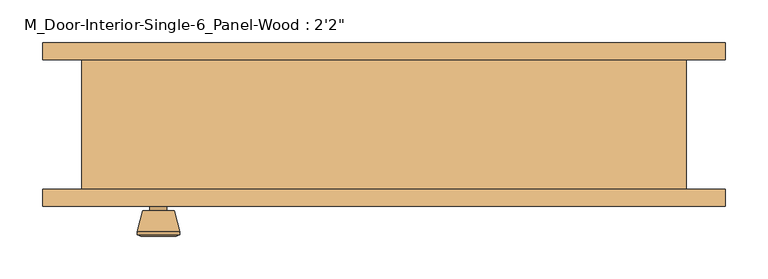
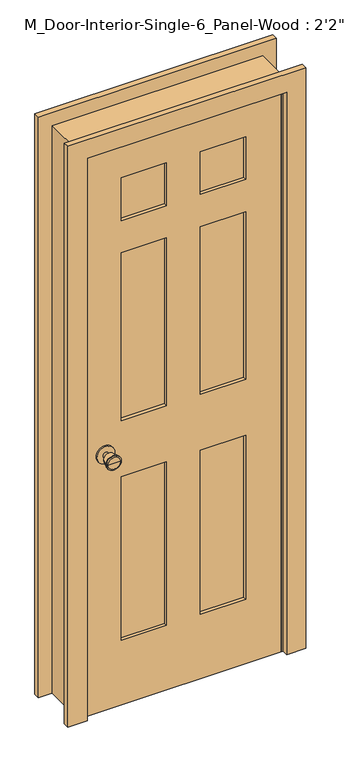
"""IFC4 building model written with IfcOpenShell, lengths in millimetres: door geometry."""

from ifc_helpers import new_model, si_unit, point, frame, frame_2d, origin, place, context, project, spatial, polyline, circle_curve, trimmed, segment, composite_curve, outline, extrude, faceted_brep, source, transform, mapped, element, save
from ifc_brep_helpers import plane_surface, cylinder_surface, revolved_surface, advanced_brep


def door_c896847d(model_context):
    return source(origin(), model_context, "Body", "SolidModel", [
        advanced_brep(
        [(-265.2, -32.025, 914.4), (-275.2, -32.025, 914.4), (-255.2, -32.025, 914.4), (-244.7241324, 16.975, 914.4), (-285.6758676, 16.975, 914.4), (-265.2, 16.975, 914.4), (-240.2, 15.1471319, 914.4), (-290.2, 15.1471319, 914.4), (-240.2, 11.6834537, 914.4), (-290.2, 11.6834537, 914.4), (-246.563764, -13.025, 914.4), (-283.836236, -13.025, 914.4), (-255.2, -13.025, 914.4), (-275.2, -13.025, 914.4)],
        [
            (0, 1),
            (1, 2, circle_curve(frame((-265.2, -32.025, 914.4), z_axis=(0.0, -1.0, 0.0), x_axis=(-1.0, 0.0, 0.0)), 10.0)),
            (2, 0),
            (2, 1, circle_curve(frame((-265.2, -32.025, 914.4), z_axis=(0.0, -1.0, 0.0), x_axis=(-1.0, 0.0, 0.0)), 10.0)),
            (3, 4, circle_curve(frame((-265.2, 16.975, 914.4), z_axis=(0.0, 1.0, 0.0), x_axis=(-1.0, 0.0, 0.0)), 20.4758676)),
            (4, 5),
            (5, 3),
            (4, 3, circle_curve(frame((-265.2, 16.975, 914.4), z_axis=(0.0, 1.0, 0.0), x_axis=(-1.0, 0.0, 0.0)), 20.4758676)),
            (6, 7, circle_curve(frame((-265.2, 15.1471319, 914.4), z_axis=(0.0, 1.0, 0.0), x_axis=(-1.0, 0.0, 0.0)), 25.0)),
            (7, 4),
            (3, 6),
            (7, 6, circle_curve(frame((-265.2, 15.1471319, 914.4), z_axis=(0.0, 1.0, 0.0), x_axis=(-1.0, 0.0, 0.0)), 25.0)),
            (8, 9, circle_curve(frame((-265.2, 11.6834537, 914.4), z_axis=(0.0, 1.0, 0.0), x_axis=(-1.0, 0.0, 0.0)), 25.0)),
            (9, 7),
            (6, 8),
            (9, 8, circle_curve(frame((-265.2, 11.6834537, 914.4), z_axis=(0.0, 1.0, 0.0), x_axis=(-1.0, 0.0, 0.0)), 25.0)),
            (10, 11, circle_curve(frame((-265.2, -13.025, 914.4), z_axis=(0.0, 1.0, 0.0), x_axis=(-1.0, 0.0, 0.0)), 18.636236)),
            (11, 9),
            (8, 10),
            (11, 10, circle_curve(frame((-265.2, -13.025, 914.4), z_axis=(0.0, 1.0, 0.0), x_axis=(-1.0, 0.0, 0.0)), 18.636236)),
            (12, 13, circle_curve(frame((-265.2, -13.025, 914.4), z_axis=(0.0, 1.0, 0.0), x_axis=(-1.0, 0.0, 0.0)), 10.0)),
            (13, 11),
            (10, 12),
            (13, 12, circle_curve(frame((-265.2, -13.025, 914.4), z_axis=(0.0, 1.0, 0.0), x_axis=(-1.0, 0.0, 0.0)), 10.0)),
            (1, 13),
            (12, 2),
        ],
        [
            plane_surface(frame((-265.2, -32.025, 914.4), z_axis=(0.0, -1.0, 0.0), x_axis=(-1.0, 0.0, 0.0))),
            plane_surface(frame((-265.2, 16.975, 914.4), z_axis=(0.0, 1.0, 0.0), x_axis=(-1.0, 0.0, 0.0))),
            revolved_surface(polyline([(-285.6758676, 16.975, 914.4), (-290.2, 15.1471319, 914.4)]), (-265.2, -32.025, 914.4), (0.0, -1.0, 0.0)),
            cylinder_surface(frame((-265.2, -32.025, 914.4), z_axis=(0.0, -1.0, 0.0), x_axis=(-1.0, 0.0, 0.0)), 25.0),
            revolved_surface(polyline([(-290.2, 11.6834537, 914.4), (-283.836236, -13.025, 914.4)]), (-265.2, -32.025, 914.4), (0.0, -1.0, 0.0)),
            plane_surface(frame((-265.2, -13.025, 914.4), z_axis=(0.0, -1.0, 0.0), x_axis=(-1.0, 0.0, 0.0))),
            cylinder_surface(frame((-265.2, -32.025, 914.4), z_axis=(0.0, -1.0, 0.0), x_axis=(-1.0, 0.0, 0.0)), 10.0),
        ],
        [
            (0, [[1, 2, 3]]),
            (0, [[-3, 4, -1]]),
            (1, [[5, 6, 7]]),
            (1, [[8, -7, -6]]),
            (2, [[9, 10, -5, 11]]),
            (2, [[12, -11, -8, -10]]),
            (3, [[13, 14, -9, 15]]),
            (3, [[16, -15, -12, -14]]),
            (4, [[17, 18, -13, 19]]),
            (4, [[20, -19, -16, -18]]),
            (5, [[21, 22, -17, 23]]),
            (5, [[24, -23, -20, -22]]),
            (6, [[-2, 25, -21, 26]]),
            (6, [[-4, -26, -24, -25]]),
        ],
    ),
        extrude(outline(composite_curve([segment(trimmed(circle_curve(frame_2d((914.4, -265.2)), 30.0), [point((914.4, -295.2))], [point((914.4, -235.2))], False, "CARTESIAN"), True, "CONTINUOUS"), segment(trimmed(circle_curve(frame_2d((914.4, -265.2)), 30.0), [point((914.4, -235.2))], [point((914.4, -295.2))], False, "CARTESIAN"), True, "CONTINUOUS")], self_intersect=False)), frame((0.0, -38.025, 0.0), z_axis=(0.0, 1.0, 0.0), x_axis=(0.0, 0.0, 1.0)), (0.0, 0.0, 1.0), 6.0),
        advanced_brep(
        [(-265.2, -79.025, 914.4), (-255.2, -79.025, 914.4), (-275.2, -79.025, 914.4), (-244.7241324, -128.025, 914.4), (-265.2, -128.025, 914.4), (-285.6758676, -128.025, 914.4), (-240.2, -126.1971319, 914.4), (-290.2, -126.1971319, 914.4), (-240.2, -122.7334537, 914.4), (-290.2, -122.7334537, 914.4), (-246.563764, -98.025, 914.4), (-283.836236, -98.025, 914.4), (-255.2, -98.025, 914.4), (-275.2, -98.025, 914.4)],
        [
            (0, 1),
            (1, 2, circle_curve(frame((-265.2, -79.025, 914.4), z_axis=(0.0, 1.0, 0.0), x_axis=(-1.0, 0.0, 0.0)), 10.0)),
            (2, 0),
            (2, 1, circle_curve(frame((-265.2, -79.025, 914.4), z_axis=(0.0, 1.0, 0.0), x_axis=(-1.0, 0.0, 0.0)), 10.0)),
            (3, 4),
            (4, 5),
            (5, 3, circle_curve(frame((-265.2, -128.025, 914.4), z_axis=(0.0, -1.0, 0.0), x_axis=(-1.0, 0.0, 0.0)), 20.4758676)),
            (3, 5, circle_curve(frame((-265.2, -128.025, 914.4), z_axis=(0.0, -1.0, 0.0), x_axis=(-1.0, 0.0, 0.0)), 20.4758676)),
            (6, 3),
            (5, 7),
            (7, 6, circle_curve(frame((-265.2, -126.1971319, 914.4), z_axis=(0.0, -1.0, 0.0), x_axis=(-1.0, 0.0, 0.0)), 25.0)),
            (6, 7, circle_curve(frame((-265.2, -126.1971319, 914.4), z_axis=(0.0, -1.0, 0.0), x_axis=(-1.0, 0.0, 0.0)), 25.0)),
            (8, 6),
            (7, 9),
            (9, 8, circle_curve(frame((-265.2, -122.7334537, 914.4), z_axis=(0.0, -1.0, 0.0), x_axis=(-1.0, 0.0, 0.0)), 25.0)),
            (8, 9, circle_curve(frame((-265.2, -122.7334537, 914.4), z_axis=(0.0, -1.0, 0.0), x_axis=(-1.0, 0.0, 0.0)), 25.0)),
            (10, 8),
            (9, 11),
            (11, 10, circle_curve(frame((-265.2, -98.025, 914.4), z_axis=(0.0, -1.0, 0.0), x_axis=(-1.0, 0.0, 0.0)), 18.636236)),
            (10, 11, circle_curve(frame((-265.2, -98.025, 914.4), z_axis=(0.0, -1.0, 0.0), x_axis=(-1.0, 0.0, 0.0)), 18.636236)),
            (12, 10),
            (11, 13),
            (13, 12, circle_curve(frame((-265.2, -98.025, 914.4), z_axis=(0.0, -1.0, 0.0), x_axis=(-1.0, 0.0, 0.0)), 10.0)),
            (12, 13, circle_curve(frame((-265.2, -98.025, 914.4), z_axis=(0.0, -1.0, 0.0), x_axis=(-1.0, 0.0, 0.0)), 10.0)),
            (1, 12),
            (13, 2),
        ],
        [
            plane_surface(frame((-265.2, -79.025, 914.4), z_axis=(0.0, 1.0, 0.0), x_axis=(-1.0, 0.0, 0.0))),
            plane_surface(frame((-265.2, -128.025, 914.4), z_axis=(0.0, -1.0, 0.0), x_axis=(-1.0, 0.0, 0.0))),
            revolved_surface(polyline([(-285.6758676, -128.025, 914.4), (-290.2, -126.1971319, 914.4)]), (-265.2, -79.025, 914.4), (0.0, 1.0, 0.0)),
            cylinder_surface(frame((-265.2, -79.025, 914.4), z_axis=(0.0, 1.0, 0.0), x_axis=(-1.0, 0.0, 0.0)), 25.0),
            revolved_surface(polyline([(-290.2, -122.7334537, 914.4), (-283.836236, -98.025, 914.4)]), (-265.2, -79.025, 914.4), (0.0, 1.0, 0.0)),
            plane_surface(frame((-265.2, -98.025, 914.4), z_axis=(0.0, 1.0, 0.0), x_axis=(-1.0, 0.0, 0.0))),
            cylinder_surface(frame((-265.2, -79.025, 914.4), z_axis=(0.0, 1.0, 0.0), x_axis=(-1.0, 0.0, 0.0)), 10.0),
        ],
        [
            (0, [[1, 2, 3]]),
            (0, [[-3, 4, -1]]),
            (1, [[5, 6, 7]]),
            (1, [[-6, -5, 8]]),
            (2, [[9, -7, 10, 11]]),
            (2, [[-10, -8, -9, 12]]),
            (3, [[13, -11, 14, 15]]),
            (3, [[-14, -12, -13, 16]]),
            (4, [[17, -15, 18, 19]]),
            (4, [[-18, -16, -17, 20]]),
            (5, [[21, -19, 22, 23]]),
            (5, [[-22, -20, -21, 24]]),
            (6, [[25, -23, 26, -2]]),
            (6, [[-26, -24, -25, -4]]),
        ],
    ),
        extrude(outline(composite_curve([segment(trimmed(circle_curve(frame_2d((914.4, -265.2)), 30.0), [point((914.4, -295.2))], [point((914.4, -235.2))], False, "CARTESIAN"), True, "CONTINUOUS"), segment(trimmed(circle_curve(frame_2d((914.4, -265.2)), 30.0), [point((914.4, -235.2))], [point((914.4, -295.2))], False, "CARTESIAN"), True, "CONTINUOUS")], self_intersect=False)), frame((0.0, -79.025, 0.0), z_axis=(0.0, 1.0, 0.0), x_axis=(0.0, 0.0, 1.0)), (0.0, 0.0, 1.0), 6.0),
        faceted_brep([(355.2, -73.025, 0.0), (330.2, -73.025, 0.0), (330.2, -38.025, 0.0), (317.5, -38.025, 0.0), (317.5, -3.1, 0.0), (330.2, -3.1, 0.0), (330.2, 79.375, 0.0), (355.2, 79.375, 0.0), (355.2, 79.375, 2025.0), (355.2, -73.025, 2025.0), (330.2, 79.375, 2000.0), (-330.2, 79.375, 2000.0), (-330.2, 79.375, 0.0), (-355.2, 79.375, 0.0), (-355.2, 79.375, 2025.0), (330.2, -3.1, 2000.0), (317.5, -3.1, 1987.3), (-317.5, -3.1, 1987.3), (-317.5, -3.1, 0.0), (-330.2, -3.1, 0.0), (-330.2, -3.1, 2000.0), (317.5, -38.025, 1987.3), (330.2, -38.025, 2000.0), (-330.2, -38.025, 2000.0), (-330.2, -38.025, 0.0), (-317.5, -38.025, 0.0), (-317.5, -38.025, 1987.3), (330.2, -73.025, 2000.0), (-355.2, -73.025, 2025.0), (-355.2, -73.025, 0.0), (-330.2, -73.025, 0.0), (-330.2, -73.025, 2000.0)], [[[0, 1, 2, 3, 4, 5, 6, 7]], [[7, 8, 9, 0]], [[6, 10, 11, 12, 13, 14, 8, 7]], [[5, 15, 10, 6]], [[4, 16, 17, 18, 19, 20, 15, 5]], [[3, 21, 16, 4]], [[2, 22, 23, 24, 25, 26, 21, 3]], [[1, 27, 22, 2]], [[0, 9, 28, 29, 30, 31, 27, 1]], [[8, 14, 28, 9]], [[15, 20, 11, 10]], [[21, 26, 17, 16]], [[27, 31, 23, 22]], [[29, 13, 12, 19, 18, 25, 24, 30]], [[14, 13, 29, 28]], [[20, 19, 12, 11]], [[26, 25, 18, 17]], [[31, 30, 24, 23]]]),
        extrude(outline(polyline([(2000.0, -330.2), (0.0, -330.2), (0.0, 330.2), (2000.0, 330.2), (2000.0, -330.2)]), holes=[polyline([(1880.0, 57.5), (1880.0, 210.2), (1727.3, 210.2), (1727.3, 57.5), (1880.0, 57.5)]), polyline([(1612.3, 210.2), (1014.4, 210.2), (1014.4, 57.5), (1612.3, 57.5), (1612.3, 210.2)]), polyline([(1014.4, -57.5), (1014.4, -210.2), (1612.3, -210.2), (1612.3, -57.5), (1014.4, -57.5)]), polyline([(1727.3, -210.2), (1880.0, -210.2), (1880.0, -57.5), (1727.3, -57.5), (1727.3, -210.2)]), polyline([(814.4, 57.5), (814.4, 210.2), (230.0, 210.2), (230.0, 57.5), (814.4, 57.5)]), polyline([(230.0, -57.5), (230.0, -210.2), (814.4, -210.2), (814.4, -57.5), (230.0, -57.5)])]), frame((0.0, -73.025, 0.0), z_axis=(0.0, 1.0, 0.0), x_axis=(0.0, 0.0, 1.0)), (0.0, 0.0, 1.0), 35.0),
        extrude(outline(polyline([(210.2, -49.6916667), (210.2, -61.3583333), (57.5, -61.3583333), (57.5, -49.6916667), (210.2, -49.6916667)])), frame((0.0, 0.0, 1727.3), z_axis=(0.0, 0.0, 1.0), x_axis=(1.0, 0.0, 0.0)), (0.0, 0.0, 1.0), 152.7),
        extrude(outline(polyline([(210.2, -49.6916667), (210.2, -61.3583333), (57.5, -61.3583333), (57.5, -49.6916667), (210.2, -49.6916667)])), frame((0.0, 0.0, 1014.4), z_axis=(0.0, 0.0, 1.0), x_axis=(1.0, 0.0, 0.0)), (0.0, 0.0, 1.0), 597.9),
        extrude(outline(polyline([(-57.5, -49.6916667), (-57.5, -61.3583333), (-210.2, -61.3583333), (-210.2, -49.6916667), (-57.5, -49.6916667)])), frame((0.0, 0.0, 1014.4), z_axis=(0.0, 0.0, 1.0), x_axis=(1.0, 0.0, 0.0)), (0.0, 0.0, 1.0), 597.9),
        extrude(outline(polyline([(-57.5, -49.6916667), (-57.5, -61.3583333), (-210.2, -61.3583333), (-210.2, -49.6916667), (-57.5, -49.6916667)])), frame((0.0, 0.0, 1727.3), z_axis=(0.0, 0.0, 1.0), x_axis=(1.0, 0.0, 0.0)), (0.0, 0.0, 1.0), 152.7),
        extrude(outline(polyline([(210.2, -49.6916667), (210.2, -61.3583333), (57.5, -61.3583333), (57.5, -49.6916667), (210.2, -49.6916667)])), frame((0.0, 0.0, 230.0), z_axis=(0.0, 0.0, 1.0), x_axis=(1.0, 0.0, 0.0)), (0.0, 0.0, 1.0), 584.4),
        extrude(outline(polyline([(-57.5, -49.6916667), (-57.5, -61.3583333), (-210.2, -61.3583333), (-210.2, -49.6916667), (-57.5, -49.6916667)])), frame((0.0, 0.0, 230.0), z_axis=(0.0, 0.0, 1.0), x_axis=(1.0, 0.0, 0.0)), (0.0, 0.0, 1.0), 584.4),
        extrude(outline(polyline([(0.0, 401.55), (2071.35, 401.55), (2071.35, -401.55), (0.0, -401.55), (0.0, -336.55), (2006.35, -336.55), (2006.35, 336.55), (0.0, 336.55), (0.0, 401.55)])), frame((0.0, -93.025, 0.0), z_axis=(0.0, 1.0, 0.0), x_axis=(0.0, 0.0, 1.0)), (0.0, 0.0, 1.0), 20.0),
        extrude(outline(polyline([(0.0, 401.55), (2071.35, 401.55), (2071.35, -401.55), (0.0, -401.55), (0.0, -336.55), (2006.35, -336.55), (2006.35, 336.55), (0.0, 336.55), (0.0, 401.55)])), frame((0.0, 79.375, 0.0), z_axis=(0.0, 1.0, 0.0), x_axis=(0.0, 0.0, 1.0)), (0.0, 0.0, 1.0), 20.0),
    ])


if __name__ == "__main__":
    model = new_model("IFC4")
    model_context = context("Model", 3, world=origin())
    ifc_project = project(units=[si_unit("LENGTHUNIT", "METRE", prefix="MILLI")], contexts=[model_context])
    site = spatial("IfcSite", under=ifc_project)
    building = spatial("IfcBuilding", under=site)
    placement = place(None, origin())
    door_shape = door_c896847d(model_context)
    element("IfcDoor", 1, ObjectType="M_Door-Interior-Single-6_Panel-Wood : 2'2\"", at=placement, inside=building, context=model_context, shape_type="MappedRepresentation", body=[
        mapped(door_shape, transform((0.0, 0.0, 0.0), x_axis=(1.0, 0.0, 0.0), y_axis=(0.0, 1.0, 0.0), z_axis=(0.0, 0.0, 1.0))),
    ])
    save(model, "model.ifc")

# Revit data of these elements
# Type "M_Door-Interior-Single-6_Panel-Wood : 2'2\""
#   Type Mark = "47"
#   Assembly Code = "C1020300"
#   Analytic Construction = "Wooden"
#   Top Rail = 0' - 4.72441"
#   Top Panel = 0' - 6.01181"
#   Thickness = 0' - 1.37795"
#   Thermal Resistance (R) = 0.455703 (m²·K)/W
#   Swing Angle [instance default] = 90.00°
#   Stiles = 0' - 4.72441"
#   Rough Width = 2' - 3.9685"
#   Rough Height = 6' - 7.72441"
#   Mullion = 0' - 4.52756"
#   Lock Rail = 0' - 7.87402"
#   Intermediate Rail = 0' - 4.52756"
#   Height = 6' - 6.74016"
#   Width = 2' - 2"
#   Heat Transfer Coefficient (U) = 2.19465 W/(m²·K)
#   Bottom Rail = 0' - 9.05512"
#   Trim Material = Cherry
#   Panel Material = Cherry
#   Frame Material = Cherry
#   Door Handle Material = Aluminum
#   Visual Light Transmittance = 0
#   Solar Heat Gain Coefficient = 0
#   Wall Closure = (empty or 0)
#   Function = (empty or 0)
# Element 1 (IfcDoor, "M_Door-Interior-Single-6_Panel-Wood : 2'2\"")
#   Materials on its faces: "Cherry", "Aluminum"
# Materials
#   "Cherry": class "Wood", colour RGB 226 177 128, transparency 0, Description = "Prunus Serotina", Cost = 0
#   "Aluminum": class "Metal", colour RGB 247 247 247, transparency 0, Description = "Aluminum 6061", Cost = 0
